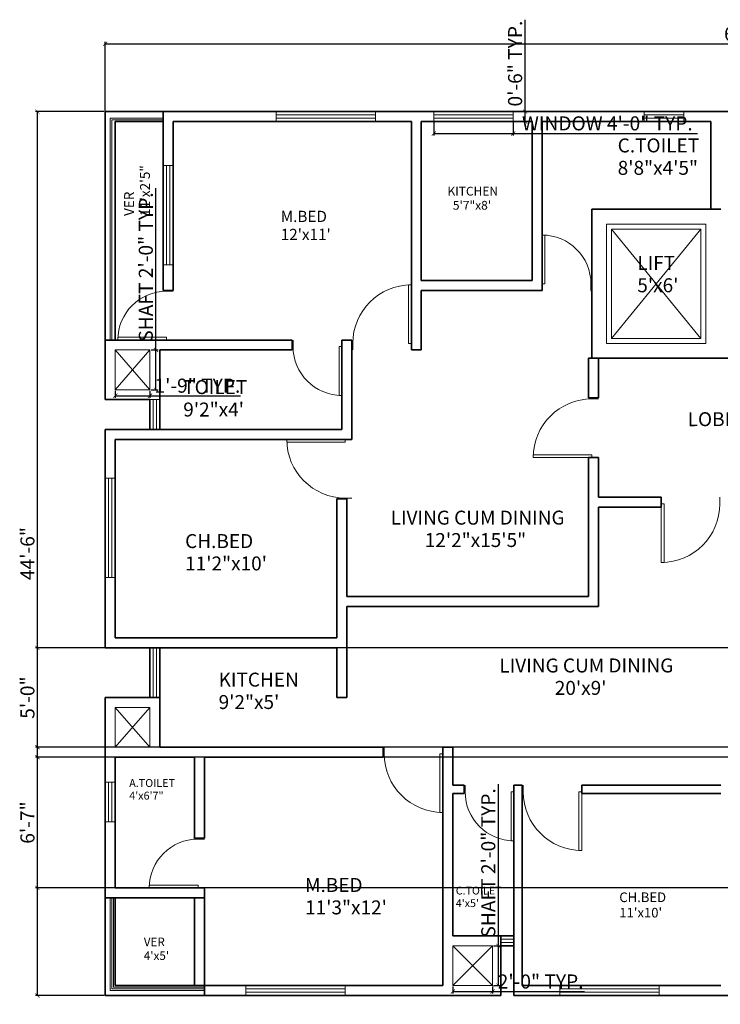
# Model space of a CAD drawing. Units: inches. Extents: x 3799 to 20199, y 1682 to 8087.
# Tile 2 of 30: x 6193 to 6616, y 1766 to 2361. Entities that reach past the tile are written whole.
import ezdxf

# ---------------------------------------------------------------- set-up
doc = ezdxf.new("R2010")
doc.units = ezdxf.units.IN
for name, color, linetype, lineweight in [('A-ANNO-DIMS', 2, 'Continuous', 18), ('A-AREA-IDEN', 7, 'Continuous', 18), ('A-DOOR', 3, 'Continuous', 18), ('A-FLOR-RAIL', 217, 'Continuous', 18), ('A-FLOR-SHFT', 8, 'Continuous', 18), ('A-GLAZ', 152, 'Continuous', 18), ('A-WALL', 7, 'Continuous', 35)]:
    doc.layers.add(name, color=color, linetype=linetype, lineweight=lineweight)
doc.styles.get("Standard").update_dxf_attribs({"font": 'arial.ttf'})
doc.dimstyles.new('ISO-25', dxfattribs={"dimtxt": 8.5, "dimasz": 2.5, "dimexe": 1.25, "dimexo": 0.625, "dimtad": 1, "dimdec": 0, "dimlunit": 3, "dimtxsty": 'Standard', "dimblk": 'ARCHTICK', "dimcen": 2.5, "dimadec": 0, "dimazin": 0, "dimtfac": 1, "dimtdec": 0, "dimtmove": 0, "dimatfit": 3, "dimfxl": 1, "dimarcsym": 0})

# ---------------------------------------------------------------- blocks, each defined once
blk = doc.blocks.new('*U7')
for p, q in [((0, 0), (0, -100)), ((750, 0), (750, -100))]:
    blk.add_line(p, q)
blk.add_lwpolyline([(0, 0), (0, 750), (43.75, 750), (43.75, 0)], close=True)
blk.add_arc((0, 0), 750, 0, 90)
blk = doc.blocks.new('*U8')
for p, q in [((0, 0), (0, -100)), ((-900, 0), (-900, -100))]:
    blk.add_line(p, q)
blk.add_lwpolyline([(0, 0), (0, 900), (-43.75, 900), (-43.75, 0)], close=True)
blk.add_arc((0, 0), 900, 90, 180)
blk = doc.blocks.new('*U9')
for p, q in [((-750, 0), (-750, 100)), ((0, 0), (0, 100))]:
    blk.add_line(p, q)
blk.add_lwpolyline([(0, 0), (0, -750), (-43.75, -750), (-43.75, 0)], close=True)
blk.add_arc((0, 0), 750, 180, 270)
blk = doc.blocks.new('*U11')
for p, q in [((-900, 0), (-900, 100)), ((0, 0), (0, 100))]:
    blk.add_line(p, q)
blk.add_lwpolyline([(0, 0), (0, -900), (-43.75, -900), (-43.75, 0)], close=True)
blk.add_arc((0, 0), 900, 180, 270)
blk = doc.blocks.new('*U10')
for p, q in [((0, 0), (0, -100)), ((900, 0), (900, -100))]:
    blk.add_line(p, q)
blk.add_lwpolyline([(0, 0), (0, 900), (43.75, 900), (43.75, 0)], close=True)
blk.add_arc((0, 0), 900, 0, 90)
blk = doc.blocks.new('*U12')
for p, q in [((0, 0), (0, -100)), ((750, 0), (750, -100))]:
    blk.add_line(p, q)
blk.add_lwpolyline([(0, 0), (0, 750), (43.75, 750), (43.75, 0)], close=True)
blk.add_arc((0, 0), 750, 0, 90)
blk = doc.blocks.new('WIN-60IN-6IN-FRAME')
for p, q in [((6, 60), (0, 60)), ((2, 60), (2, 0)), ((4, 60), (4, 0)), ((6, 0), (0, 0))]:
    blk.add_line(p, q)
blk = doc.blocks.new('WIN-24IN-6IN-FRAME')
for p, q in [((6, 24), (0, 24)), ((2, 24), (2, 0)), ((4, 24), (4, 0)), ((6, 0), (0, 0))]:
    blk.add_line(p, q)
blk = doc.blocks.new('WIN-48IN-6IN-FRAME')
for p, q in [((0, 0), (0, 6)), ((48, 0), (48, 6)), ((48, 4), (0, 4)), ((48, 2), (0, 2))]:
    blk.add_line(p, q)
blk = doc.blocks.new('SHAFT-21X24IN')
for p, q in [((0, 24), (0, 0)), ((21, 24), (0, 24)), ((0, 24), (21, 0)), ((21, 24), (0, 0)), ((21, 24), (21, 0)), ((21, 0), (0, 0))]:
    blk.add_line(p, q)
blk = doc.blocks.new('SHAFT-24X24IN')
for p, q in [((0, 24), (0, 0)), ((24, 24), (0, 24)), ((0, 24), (24, 0)), ((0, 0), (24, 24)), ((24, 24), (24, 0)), ((0, 0), (24, 0))]:
    blk.add_line(p, q)
blk = doc.blocks.new('_ArchTick')
at = {"color": 0, "linetype": 'ByBlock', "const_width": 0.15}
blk.add_lwpolyline([(-0.5, -0.5), (0.5, 0.5)], dxfattribs=at)
blk = doc.blocks.new('*D302')
at = {"layer": 'A-ANNO-DIMS', "color": 0, "lineweight": -2, "transparency": 16777216}
for p, q in [((6443.22, 2298.42), (6443.22, 2290.6)), ((6491.22, 2298.42), (6491.22, 2290.6)), ((6443.22, 2291.85), (6491.22, 2291.85)), ((6491.22, 2291.85), (6602.53, 2291.85))]:
    blk.add_line(p, q, dxfattribs=at)
at = {"layer": 'Defpoints', "color": 0, "transparency": 16777216}
for p in [(6443.22, 2299.05), (6491.22, 2299.05), (6491.22, 2291.85)]:
    blk.add_point(p, dxfattribs=at)
at = {"layer": 'A-ANNO-DIMS', "color": 0, "lineweight": -2, "transparency": 16777216, "xscale": 2.5, "yscale": 2.5, "zscale": 2.5, "rotation": 180}
blk.add_blockref('_ArchTick', (6443.22, 2291.85), dxfattribs=at)
at = {"layer": 'A-ANNO-DIMS', "color": 0, "lineweight": -2, "transparency": 16777216, "xscale": 2.5, "yscale": 2.5, "zscale": 2.5}
blk.add_blockref('_ArchTick', (6491.22, 2291.85), dxfattribs=at)
at = {"layer": 'A-ANNO-DIMS', "color": 0, "transparency": 16777216, "insert": (6548.12, 2296.87), "char_height": 8.5, "attachment_point": 5}
blk.add_mtext('WINDOW 4\'-0" TYP.', dxfattribs=at)
blk = doc.blocks.new('*D303')
at = {"layer": 'A-ANNO-DIMS', "color": 0, "lineweight": -2, "transparency": 16777216}
for p, q in [((6498.42, 2305.05), (6498.42, 2360.61)), ((6491.84, 2305.05), (6499.67, 2305.05)), ((6498.42, 2299.05), (6498.42, 2305.05)), ((6491.84, 2299.05), (6499.67, 2299.05))]:
    blk.add_line(p, q, dxfattribs=at)
at = {"layer": 'Defpoints', "color": 0, "transparency": 16777216}
for p in [(6491.22, 2305.05), (6498.42, 2305.05), (6491.22, 2299.05)]:
    blk.add_point(p, dxfattribs=at)
at = {"layer": 'A-ANNO-DIMS', "color": 0, "lineweight": -2, "transparency": 16777216, "xscale": 2.5, "yscale": 2.5, "zscale": 2.5}
for p, rotation in [((6498.42, 2305.05), 90), ((6498.42, 2299.05), 270)]:
    blk.add_blockref('_ArchTick', p, dxfattribs=dict(at, rotation=rotation))
at = {"layer": 'A-ANNO-DIMS', "color": 0, "transparency": 16777216, "insert": (6493.45, 2334.08), "char_height": 8.5, "attachment_point": 5, "rotation": 90}
blk.add_mtext('0\'-6" TYP.', dxfattribs=at)
blk = doc.blocks.new('*D342')
at = {"layer": 'A-ANNO-DIMS', "color": 0, "lineweight": -2, "transparency": 16777216}
for p, q in [((6275.27, 2161.05), (6275.27, 2258.79)), ((6272.3, 2161.05), (6276.52, 2161.05)), ((6275.27, 2137.05), (6275.27, 2161.05)), ((6272.3, 2137.05), (6276.52, 2137.05))]:
    blk.add_line(p, q, dxfattribs=at)
at = {"layer": 'Defpoints', "color": 0, "transparency": 16777216}
for p in [(6271.67, 2161.05), (6275.27, 2161.05), (6271.67, 2137.05)]:
    blk.add_point(p, dxfattribs=at)
at = {"layer": 'A-ANNO-DIMS', "color": 0, "lineweight": -2, "transparency": 16777216, "xscale": 2.5, "yscale": 2.5, "zscale": 2.5}
for p, rotation in [((6275.27, 2161.05), 90), ((6275.27, 2137.05), 270)]:
    blk.add_blockref('_ArchTick', p, dxfattribs=dict(at, rotation=rotation))
at = {"layer": 'A-ANNO-DIMS', "color": 0, "transparency": 16777216, "insert": (6270.25, 2211.17), "char_height": 8.5, "attachment_point": 5, "rotation": 90}
blk.add_mtext('SHAFT 2\'-0" TYP.', dxfattribs=at)
blk = doc.blocks.new('*D343')
at = {"layer": 'A-ANNO-DIMS', "color": 0, "lineweight": -2, "transparency": 16777216}
for p, q in [((6250.67, 2136.42), (6250.67, 2132.2)), ((6271.67, 2136.42), (6271.67, 2132.2)), ((6250.67, 2133.45), (6271.67, 2133.45)), ((6271.67, 2133.45), (6326.44, 2133.45))]:
    blk.add_line(p, q, dxfattribs=at)
at = {"layer": 'Defpoints', "color": 0, "transparency": 16777216}
for p in [(6250.67, 2137.05), (6271.67, 2137.05), (6271.67, 2133.45)]:
    blk.add_point(p, dxfattribs=at)
at = {"layer": 'A-ANNO-DIMS', "color": 0, "lineweight": -2, "transparency": 16777216, "xscale": 2.5, "yscale": 2.5, "zscale": 2.5, "rotation": 180}
blk.add_blockref('_ArchTick', (6250.67, 2133.45), dxfattribs=at)
at = {"layer": 'A-ANNO-DIMS', "color": 0, "lineweight": -2, "transparency": 16777216, "xscale": 2.5, "yscale": 2.5, "zscale": 2.5}
blk.add_blockref('_ArchTick', (6271.67, 2133.45), dxfattribs=at)
at = {"layer": 'A-ANNO-DIMS', "color": 0, "transparency": 16777216, "insert": (6300.31, 2138.41), "char_height": 8.5, "attachment_point": 5}
blk.add_mtext('1\'-9" TYP.', dxfattribs=at)
blk = doc.blocks.new('*D344')
at = {"layer": 'A-ANNO-DIMS', "color": 0, "lineweight": -2, "transparency": 16777216}
for p, q in [((6482.27, 1801.05), (6482.27, 1898.79)), ((6479.3, 1801.05), (6483.52, 1801.05)), ((6482.27, 1777.05), (6482.27, 1801.05)), ((6479.3, 1777.05), (6483.52, 1777.05))]:
    blk.add_line(p, q, dxfattribs=at)
at = {"layer": 'Defpoints', "color": 0, "transparency": 16777216}
for p in [(6478.67, 1801.05), (6482.27, 1801.05), (6478.67, 1777.05)]:
    blk.add_point(p, dxfattribs=at)
at = {"layer": 'A-ANNO-DIMS', "color": 0, "lineweight": -2, "transparency": 16777216, "xscale": 2.5, "yscale": 2.5, "zscale": 2.5}
for p, rotation in [((6482.27, 1801.05), 90), ((6482.27, 1777.05), 270)]:
    blk.add_blockref('_ArchTick', p, dxfattribs=dict(at, rotation=rotation))
at = {"layer": 'A-ANNO-DIMS', "color": 0, "transparency": 16777216, "insert": (6477.25, 1851.17), "char_height": 8.5, "attachment_point": 5, "rotation": 90}
blk.add_mtext('SHAFT 2\'-0" TYP.', dxfattribs=at)
blk = doc.blocks.new('*D345')
at = {"layer": 'A-ANNO-DIMS', "color": 0, "lineweight": -2, "transparency": 16777216}
for p, q in [((6454.67, 1776.42), (6454.67, 1772.2)), ((6454.67, 1773.45), (6478.67, 1773.45)), ((6478.67, 1776.42), (6478.67, 1772.2)), ((6478.67, 1773.45), (6534.38, 1773.45))]:
    blk.add_line(p, q, dxfattribs=at)
at = {"layer": 'Defpoints', "color": 0, "transparency": 16777216}
for p in [(6454.67, 1777.05), (6478.67, 1777.05), (6478.67, 1773.45)]:
    blk.add_point(p, dxfattribs=at)
at = {"layer": 'A-ANNO-DIMS', "color": 0, "lineweight": -2, "transparency": 16777216, "xscale": 2.5, "yscale": 2.5, "zscale": 2.5, "rotation": 180}
blk.add_blockref('_ArchTick', (6454.67, 1773.45), dxfattribs=at)
at = {"layer": 'A-ANNO-DIMS', "color": 0, "lineweight": -2, "transparency": 16777216, "xscale": 2.5, "yscale": 2.5, "zscale": 2.5}
blk.add_blockref('_ArchTick', (6478.67, 1773.45), dxfattribs=at)
at = {"layer": 'A-ANNO-DIMS', "color": 0, "transparency": 16777216, "insert": (6507.78, 1778.41), "char_height": 8.5, "attachment_point": 5}
blk.add_mtext('2\'-0" TYP.', dxfattribs=at)
blk = doc.blocks.new('*D356')
at = {"layer": 'A-ANNO-DIMS', "color": 0, "lineweight": -2, "transparency": 16777216}
for p, q in [((6244.67, 2305.67), (6244.67, 2347.3)), ((6244.67, 2346.05), (7024.67, 2346.05)), ((7024.67, 2305.67), (7024.67, 2347.3))]:
    blk.add_line(p, q, dxfattribs=at)
at = {"layer": 'Defpoints', "color": 0, "transparency": 16777216}
for p in [(7024.67, 2346.05), (6244.67, 2305.05), (7024.67, 2305.05)]:
    blk.add_point(p, dxfattribs=at)
at = {"layer": 'A-ANNO-DIMS', "color": 0, "lineweight": -2, "transparency": 16777216, "xscale": 2.5, "yscale": 2.5, "zscale": 2.5, "rotation": 180}
blk.add_blockref('_ArchTick', (6244.67, 2346.05), dxfattribs=at)
at = {"layer": 'A-ANNO-DIMS', "color": 0, "lineweight": -2, "transparency": 16777216, "xscale": 2.5, "yscale": 2.5, "zscale": 2.5}
blk.add_blockref('_ArchTick', (7024.67, 2346.05), dxfattribs=at)
at = {"layer": 'A-ANNO-DIMS', "color": 0, "transparency": 16777216, "insert": (6634.67, 2351.01), "char_height": 8.5, "attachment_point": 5}
blk.add_mtext('65\'-0"', dxfattribs=at)
blk = doc.blocks.new('*D357')
at = {"layer": 'A-ANNO-DIMS', "color": 0, "lineweight": -2, "transparency": 16777216}
for p, q in [((6244.05, 2305.05), (6202.42, 2305.05)), ((6203.67, 1771.05), (6203.67, 2305.05)), ((6244.05, 1771.05), (6202.42, 1771.05))]:
    blk.add_line(p, q, dxfattribs=at)
at = {"layer": 'Defpoints', "color": 0, "transparency": 16777216}
for p in [(6203.67, 2305.05), (6244.67, 2305.05), (6244.67, 1771.05)]:
    blk.add_point(p, dxfattribs=at)
at = {"layer": 'A-ANNO-DIMS', "color": 0, "lineweight": -2, "transparency": 16777216, "xscale": 2.5, "yscale": 2.5, "zscale": 2.5}
for p, rotation in [((6203.67, 2305.05), 90), ((6203.67, 1771.05), 270)]:
    blk.add_blockref('_ArchTick', p, dxfattribs=dict(at, rotation=rotation))
at = {"layer": 'A-ANNO-DIMS', "color": 0, "transparency": 16777216, "insert": (6198.71, 2038.05), "char_height": 8.5, "attachment_point": 5, "rotation": 90}
blk.add_mtext('44\'-6"', dxfattribs=at)
blk = doc.blocks.new('*D368')
at = {"layer": 'A-ANNO-DIMS', "color": 0, "lineweight": -2, "transparency": 16777216}
for p, q in [((6989.05, 1981.05), (6202.42, 1981.05)), ((6203.67, 1921.05), (6203.67, 1981.05)), ((6989.05, 1921.05), (6202.42, 1921.05))]:
    blk.add_line(p, q, dxfattribs=at)
at = {"layer": 'Defpoints', "color": 0, "transparency": 16777216}
for p in [(6203.67, 1981.05), (6989.67, 1981.05), (6989.67, 1921.05)]:
    blk.add_point(p, dxfattribs=at)
at = {"layer": 'A-ANNO-DIMS', "color": 0, "lineweight": -2, "transparency": 16777216, "xscale": 2.5, "yscale": 2.5, "zscale": 2.5}
for p, rotation in [((6203.67, 1981.05), 90), ((6203.67, 1921.05), 270)]:
    blk.add_blockref('_ArchTick', p, dxfattribs=dict(at, rotation=rotation))
at = {"layer": 'A-ANNO-DIMS', "color": 0, "transparency": 16777216, "insert": (6198.71, 1951.05), "char_height": 8.5, "attachment_point": 5, "rotation": 90}
blk.add_mtext('5\'-0"', dxfattribs=at)
blk = doc.blocks.new('*D370')
at = {"layer": 'A-ANNO-DIMS', "color": 0, "lineweight": -2, "transparency": 16777216}
for p, q in [((7018.05, 1915.05), (6202.42, 1915.05)), ((6203.67, 1836.05), (6203.67, 1915.05)), ((7018.05, 1836.05), (6202.42, 1836.05))]:
    blk.add_line(p, q, dxfattribs=at)
at = {"layer": 'Defpoints', "color": 0, "transparency": 16777216}
for p in [(6203.67, 1915.05), (7018.67, 1915.05), (7018.67, 1836.05)]:
    blk.add_point(p, dxfattribs=at)
at = {"layer": 'A-ANNO-DIMS', "color": 0, "lineweight": -2, "transparency": 16777216, "xscale": 2.5, "yscale": 2.5, "zscale": 2.5}
for p, rotation in [((6203.67, 1915.05), 90), ((6203.67, 1836.05), 270)]:
    blk.add_blockref('_ArchTick', p, dxfattribs=dict(at, rotation=rotation))
at = {"layer": 'A-ANNO-DIMS', "color": 0, "transparency": 16777216, "insert": (6198.71, 1875.55), "char_height": 8.5, "attachment_point": 5, "rotation": 90}
blk.add_mtext('6\'-7"', dxfattribs=at)

msp = doc.modelspace()

# ---------------------------------------------------------------- linework, layer by layer
at = {"layer": 'A-FLOR-RAIL'}
for p, q in [((6247.67, 2301.05), (6247.67, 2167.05)), ((6279.67, 2301.05), (6247.67, 2301.05)), ((6248.67, 2300.05), (6248.67, 2167.05)), ((6279.67, 2300.05), (6248.67, 2300.05)), ((6247.67, 1830.05), (6247.67, 1774.05)), ((6248.67, 1830.05), (6248.67, 1775.05)), ((6249.67, 1830.05), (6249.67, 1776.05)), ((6247.67, 1774.05), (6304.67, 1774.05)), ((6248.67, 1775.05), (6304.67, 1775.05)), ((6249.67, 1776.05), (6304.67, 1776.05)), ((6250.67, 1775.05), (6304.67, 1775.05))]:
    msp.add_line(p, q, dxfattribs=at)
at = {"layer": 'A-FLOR-SHFT'}
for p, q in [((6607.67, 2237.05), (6547.67, 2237.05)), ((6547.67, 2237.05), (6547.67, 2165.05)), ((6607.67, 2237.05), (6607.67, 2165.05)), ((6604.67, 2234.05), (6550.67, 2234.05)), ((6550.67, 2234.05), (6550.67, 2168.05)), ((6550.67, 2234.05), (6604.67, 2168.05)), ((6550.67, 2168.05), (6604.67, 2234.05)), ((6604.67, 2234.05), (6604.67, 2168.05)), ((6604.67, 2168.05), (6550.67, 2168.05)), ((6607.67, 2165.05), (6547.67, 2165.05))]:
    msp.add_line(p, q, dxfattribs=at)
at = {"layer": 'A-GLAZ'}
for p, q in [((6271.67, 2131.05), (6277.67, 2131.05)), ((6273.67, 2131.05), (6273.67, 2113.05)), ((6275.67, 2131.05), (6275.67, 2113.05)), ((6273.67, 1981.05), (6273.67, 1951.05)), ((6275.67, 1981.05), (6275.67, 1951.05)), ((6491.67, 1805.05), (6483.67, 1805.05)), ((6491.67, 1803.05), (6483.67, 1803.05))]:
    msp.add_line(p, q, dxfattribs=at)
at = {"layer": 'A-WALL'}
for p, q in [((7024.67, 2305.05), (6244.67, 2305.05)), ((6244.67, 2305.05), (6244.67, 2131.05)), ((6279.67, 2305.05), (6279.67, 2197.05)), ((6250.67, 2299.05), (6250.67, 2167.05)), ((6279.67, 2299.05), (6250.67, 2299.05)), ((6285.67, 2299.05), (6285.67, 2197.05)), ((6429.67, 2299.05), (6285.67, 2299.05)), ((6429.67, 2299.05), (6429.67, 2161.05)), ((6435.67, 2299.05), (6435.67, 2203.05)), ((6502.67, 2299.05), (6435.67, 2299.05)), ((6502.67, 2299.05), (6502.67, 2203.05)), ((6508.67, 2299.05), (6508.67, 2197.05)), ((6610.67, 2299.05), (6508.67, 2299.05)), ((6610.67, 2246.05), (6610.67, 2299.05)), ((6538.67, 2246.05), (6538.67, 2156.05)), ((6616.67, 2246.05), (6538.67, 2246.05)), ((6502.67, 2203.05), (6435.67, 2203.05)), ((6285.67, 2197.05), (6279.67, 2197.05)), ((6502.67, 2197.05), (6435.67, 2197.05)), ((6435.67, 2197.05), (6435.67, 2161.05)), ((6502.67, 2197.05), (6508.67, 2197.05)), ((6538.2, 2197.05), (6538.67, 2197.05)), ((6357.67, 2167.05), (6244.67, 2167.05)), ((6357.67, 2167.05), (6357.67, 2161.05)), ((6393.67, 2167.05), (6387.67, 2167.05)), ((6387.67, 2167.05), (6387.67, 2113.05)), ((6393.67, 2167.05), (6393.67, 2161.05)), ((6357.67, 2161.05), (6277.67, 2161.05)), ((6277.67, 2161.05), (6277.67, 2113.05)), ((6393.67, 2161.05), (6393.67, 2107.05)), ((6435.67, 2161.05), (6429.67, 2161.05)), ((6536.67, 2156.05), (6536.67, 2132.05)), ((6536.67, 2156.05), (6693.67, 2156.05)), ((6542.67, 2156.05), (6542.67, 2132.05)), ((6271.67, 2131.05), (6244.67, 2131.05)), ((6271.67, 2131.05), (6271.67, 2113.05)), ((6542.67, 2132.05), (6536.67, 2132.05)), ((6387.67, 2113.05), (6244.67, 2113.05)), ((6244.67, 2113.05), (6244.67, 1981.05)), ((6393.67, 2107.05), (6250.67, 2107.05)), ((6250.67, 2107.05), (6250.67, 1987.05)), ((6542.67, 2096.05), (6536.67, 2096.05)), ((6536.67, 2096.05), (6536.67, 2012.05)), ((6542.67, 2096.05), (6542.67, 2072.05)), ((6384.67, 2071.05), (6384.67, 1987.05)), ((6390.67, 2071.05), (6384.67, 2071.05)), ((6390.67, 2071.05), (6390.67, 2012.05)), ((6542.67, 2072.05), (6580.67, 2072.05)), ((6580.67, 2072.05), (6580.67, 2066.05)), ((6542.67, 2066.05), (6580.67, 2066.05)), ((6542.67, 2066.05), (6542.67, 2006.05)), ((6536.67, 2012.05), (6390.67, 2012.05)), ((6542.67, 2006.05), (6390.67, 2006.05)), ((6390.67, 2006.05), (6390.67, 1951.05)), ((6384.67, 1987.05), (6250.67, 1987.05)), ((6384.67, 1981.05), (6244.67, 1981.05)), ((6271.67, 1981.05), (6271.67, 1951.05)), ((6277.67, 1981.05), (6277.67, 1921.05)), ((6384.67, 1981.05), (6384.67, 1951.05)), ((6244.67, 1951.05), (6244.67, 1771.05)), ((6277.67, 1951.05), (6244.67, 1951.05)), ((6384.67, 1951.05), (6390.67, 1951.05)), ((6384.67, 1921.05), (6277.67, 1921.05)), ((6277.67, 1921.05), (6412.67, 1921.05)), ((6412.67, 1921.05), (6412.67, 1915.05)), ((6448.67, 1921.05), (6448.67, 1777.05)), ((6448.67, 1921.05), (6454.67, 1921.05)), ((6454.67, 1921.05), (6454.67, 1898.05)), ((6250.67, 1915.05), (6250.67, 1836.05)), ((6298.67, 1915.05), (6250.67, 1915.05)), ((6298.67, 1915.05), (6298.67, 1866.05)), ((6412.67, 1915.05), (6304.67, 1915.05)), ((6304.67, 1915.05), (6304.67, 1866.05)), ((6461.67, 1898.05), (6454.67, 1898.05)), ((6461.67, 1898.05), (6461.67, 1893.05)), ((6491.67, 1898.05), (6491.67, 1771.05)), ((6496.67, 1898.05), (6491.67, 1898.05)), ((6496.67, 1898.05), (6496.67, 1777.05)), ((6616.67, 1898.05), (6532.67, 1898.05)), ((6532.67, 1898.05), (6532.67, 1893.05)), ((6454.67, 1893.05), (6454.67, 1807.05)), ((6461.67, 1893.05), (6454.67, 1893.05)), ((6616.67, 1893.05), (6532.67, 1893.05)), ((6304.67, 1866.05), (6298.67, 1866.05)), ((6304.67, 1836.05), (6250.67, 1836.05)), ((6304.67, 1836.05), (6304.67, 1771.05)), ((6304.67, 1830.05), (6244.67, 1830.05)), ((6250.67, 1830.05), (6250.67, 1777.05)), ((6298.67, 1830.05), (6298.67, 1777.05)), ((6491.67, 1807.05), (6454.67, 1807.05)), ((6483.67, 1807.05), (6483.67, 1771.05)), ((6491.67, 1801.05), (6483.67, 1801.05)), ((6250.67, 1777.05), (6448.67, 1777.05)), ((6496.67, 1777.05), (6616.67, 1777.05)), ((6244.67, 1771.05), (6483.67, 1771.05)), ((6491.67, 1771.05), (6760.67, 1771.05))]:
    msp.add_line(p, q, dxfattribs=at)

# ---------------------------------------------------------------- block references
at = {"layer": 'A-DOOR', "yscale": 0.0393700787401575, "zscale": 0.0393700787401575}
for name, p, xscale in [('*U7', (6508.67, 2200.99), 0.0393700787401575), ('*U8', (6429.67, 2164.99), 0.0393700787401575), ('*U9', (6387.67, 2163.11), 0.0393700787401575), ('*U11', (6580.67, 2068.11), -0.0393700787401575), ('*U11', (6448.67, 1917.11), 0.0393700787401575), ('*U9', (6491.67, 1894.11), 0.0393700787401575), ('*U11', (6532.67, 1894.11), 0.0393700787401575)]:
    msp.add_blockref(name, p, dxfattribs=dict(at, xscale=xscale))
at = {"layer": 'A-DOOR', "xscale": 0.0393700787401575, "yscale": 0.0393700787401575, "zscale": 0.0393700787401575, "rotation": 90}
for name, p in [('*U7', (6281.74, 2167.05)), ('*U10', (6538.74, 2096.05)), ('*U8', (6389.74, 2107.05)), ('*U12', (6300.74, 1836.05))]:
    msp.add_blockref(name, p, dxfattribs=at)
at = {"layer": 'A-FLOR-SHFT'}
for name, p in [('SHAFT-21X24IN', (6250.67, 2137.05)), ('SHAFT-21X24IN', (6250.67, 1921.05)), ('SHAFT-24X24IN', (6454.68, 1777.05))]:
    msp.add_blockref(name, p, dxfattribs=at)
at = {"layer": 'A-GLAZ', "rotation": 90}
for name, p in [('WIN-60IN-6IN-FRAME', (6407.9, 2299.05)), ('WIN-24IN-6IN-FRAME', (6594.34, 2299.05)), ('WIN-60IN-6IN-FRAME', (6389.59, 1771.05)), ('WIN-60IN-6IN-FRAME', (6579.37, 1771.05))]:
    msp.add_blockref(name, p, dxfattribs=at)
at = {"layer": 'A-GLAZ'}
for name, p in [('WIN-48IN-6IN-FRAME', (6443.22, 2299.05)), ('WIN-60IN-6IN-FRAME', (6279.68, 2212.42)), ('WIN-60IN-6IN-FRAME', (6244.68, 2023.53)), ('WIN-24IN-6IN-FRAME', (6244.68, 1875.93))]:
    msp.add_blockref(name, p, dxfattribs=at)

# ---------------------------------------------------------------- texts
at = {"layer": 'A-AREA-IDEN'}
for s, height, rotation, p in [('C.TOILET', 8.428, 0.03333, (6554.35, 2280.42)), ('8\'8"x4\'5"', 8.428, 0.03333, (6554.36, 2266.88)), ('11\'x2\'5"', 5.992, 90.03333, (6271.66, 2242.06)), ('VER', 5.992, 90.03333, (6262.04, 2242.05)), ('KITCHEN', 5.306, 0.03333, (6451.51, 2254.34)), ('  5\'7"x8\'', 5.306, 0.03333, (6451.51, 2245.82)), ('M.BED', 6.77, 0.03333, (6350.7, 2238.37)), ("12'x11'", 6.77, 0.03333, (6350.7, 2227.49)), ('LIFT', 8.428, 0.03333, (6566.21, 2209.47)), ("5'x6'", 8.428, 0.03333, (6566.21, 2195.93)), ('TOILET', 8.428, 0.03333, (6291.78, 2134.4)), ('9\'2"x4\'', 8.428, 0.03333, (6291.78, 2120.86)), ('LOBBY', 8.428, 0.03333, (6596.66, 2115.03)), ('LIVING CUM DINING', 8.4277, 0.03333, (6417.12, 2055.52)), ('CH.BED', 8.428, 0.03333, (6292.91, 2041.38)), ('        12\'2"x15\'5"', 8.4277, 0.03333, (6417.13, 2041.98)), ('11\'2"x10\'', 8.428, 0.03333, (6292.92, 2027.85)), ('LIVING CUM DINING', 8.4277, 0.03333, (6482.85, 1966.2)), ('KITCHEN', 8.428, 0.03333, (6313.14, 1957.67)), ("             20'x9'", 8.4277, 0.03333, (6482.86, 1952.66)), ('9\'2"x5\'', 8.428, 0.03333, (6313.15, 1944.14)), ('A.TOILET', 4.765, 0.03333, (6259.14, 1897.05)), ('4\'x6\'7"', 4.765, 0.03333, (6259.14, 1889.4)), ('M.BED', 8.428, 0.03333, (6365.4, 1833.6)), ('C.TOILET', 4.733, 0.03333, (6456.51, 1832.07)), ('CH.BED', 5.798, 0.03333, (6555.33, 1827.5)), ('11\'3"x12\'', 8.428, 0.03333, (6365.41, 1820.06)), ("4'x5'", 4.733, 0.03333, (6456.51, 1824.47)), ("11'x10'", 5.798, 0.03333, (6555.34, 1818.19)), ('VER', 5.177, 0.03333, (6267.94, 1800.86)), ("4'x5'", 5.177, 0.03333, (6267.95, 1792.54))]:
    msp.add_text(s, height=height, rotation=rotation, dxfattribs=at).set_placement(p)

# ---------------------------------------------------------------- dimensions: what is measured, and where the dimension line sits
at = {"layer": 'A-ANNO-DIMS'}
dim = msp.add_linear_dim(base=(7024.67, 2346.05), p1=(6244.67, 2305.05), p2=(7024.67, 2305.05), dimstyle='ISO-25', override={"dimdec": 1, "dimlfac": 1, "dimrnd": 0, "dimzin": 1, "dimdsep": 46, "dimlunit": 4, "dimfrac": 2}, dxfattribs=at)
dim.commit()
dim.dimension.update_dxf_attribs({"geometry": '*D356', "text_midpoint": (6634.67, 2351.01)})
for base, p1, p2, text, picture, middle in [((6498.42, 2305.05), (6491.22, 2299.05), (6491.22, 2305.05), '<> TYP.', '*D303', (6493.45, 2334.08)), ((6275.27, 2161.05), (6271.67, 2137.05), (6271.67, 2161.05), 'SHAFT <> TYP.', '*D342', (6270.25, 2211.17)), ((6482.27, 1801.05), (6478.67, 1777.05), (6478.67, 1801.05), 'SHAFT <> TYP.', '*D344', (6477.25, 1851.17))]:
    dim = msp.add_linear_dim(base=base, p1=p1, p2=p2, angle=90, text=text, dimstyle='ISO-25', override={"dimdec": 1, "dimlfac": 1, "dimrnd": 0, "dimzin": 1, "dimdsep": 46, "dimlunit": 4, "dimfrac": 2}, dxfattribs=at)
    dim.commit()
    dim.dimension.update_dxf_attribs({"geometry": picture, "text_midpoint": middle})
for base, p1, p2, text, picture, middle in [((6491.22, 2291.85), (6443.22, 2299.05), (6491.22, 2299.05), 'WINDOW <> TYP.', '*D302', (6548.12, 2296.87)), ((6271.67, 2133.45), (6250.67, 2137.05), (6271.67, 2137.05), '<> TYP.', '*D343', (6300.31, 2138.41)), ((6478.67, 1773.45), (6454.67, 1777.05), (6478.67, 1777.05), '<> TYP.', '*D345', (6507.78, 1778.41))]:
    dim = msp.add_linear_dim(base=base, p1=p1, p2=p2, text=text, dimstyle='ISO-25', override={"dimdec": 1, "dimlfac": 1, "dimrnd": 0, "dimzin": 1, "dimdsep": 46, "dimlunit": 4, "dimfrac": 2}, dxfattribs=at)
    dim.commit()
    dim.dimension.update_dxf_attribs({"geometry": picture, "text_midpoint": middle})
for base, p1, p2, picture, middle in [((6203.67, 2305.05), (6244.67, 1771.05), (6244.67, 2305.05), '*D357', (6198.71, 2038.05)), ((6203.67, 1981.05), (6989.67, 1921.05), (6989.67, 1981.05), '*D368', (6198.71, 1951.05)), ((6203.67, 1915.05), (7018.67, 1836.05), (7018.67, 1915.05), '*D370', (6198.71, 1875.55))]:
    dim = msp.add_linear_dim(base=base, p1=p1, p2=p2, angle=90, dimstyle='ISO-25', override={"dimdec": 1, "dimlfac": 1, "dimrnd": 0, "dimzin": 1, "dimdsep": 46, "dimlunit": 4, "dimfrac": 2}, dxfattribs=at)
    dim.commit()
    dim.dimension.update_dxf_attribs({"geometry": picture, "text_midpoint": middle})

doc.saveas('drawing.dxf')
